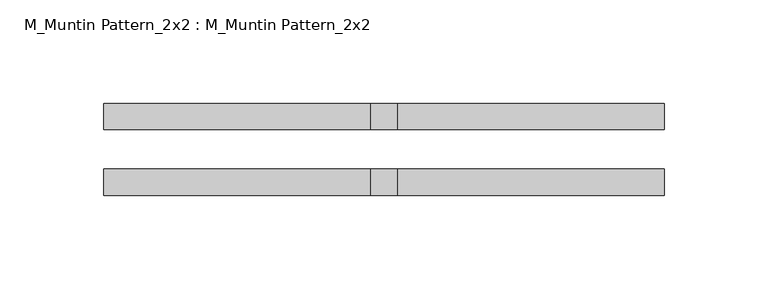
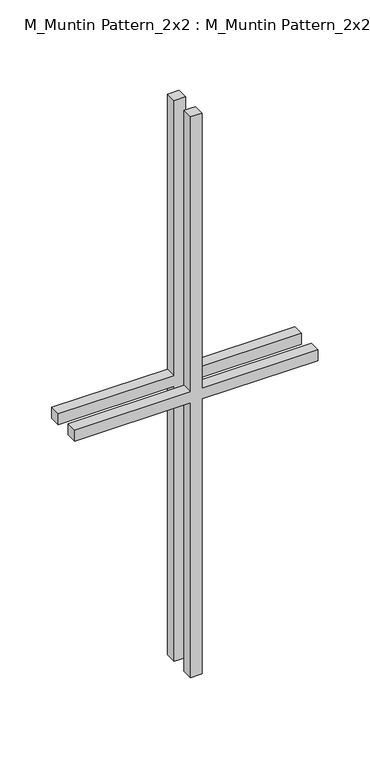
"""IFC4 building model written with IfcOpenShell, lengths in millimetres: proxy geometry, M_Muntin Pattern_2x2 : M_Muntin Pattern_2x2."""

from ifc_helpers import new_model, si_unit, frame, origin, place, context, project, spatial, polyline, outline, extrude, source, transform, mapped, element, save


def m_muntin_pattern_2x2_m_muntin_pattern_2x2_fa3d06ac(model_context):
    return source(origin(), model_context, "Body", "SweptSolid", [
        extrude(outline(polyline([(336.5, -6.35), (336.5, -135.4666667), (323.8, -135.4666667), (323.8, -6.35), (0.0, -6.35), (0.0, 6.35), (323.8, 6.35), (323.8, 135.4666667), (336.5, 135.4666667), (336.5, 6.35), (660.3, 6.35), (660.3, -6.35), (336.5, -6.35)])), frame((0.0, -22.225, 0.0), z_axis=(0.0, 1.0, 0.0), x_axis=(0.0, 0.0, 1.0)), (0.0, 0.0, 1.0), 12.7),
        extrude(outline(polyline([(336.5, -6.35), (336.5, -135.4666667), (323.8, -135.4666667), (323.8, -6.35), (0.0, -6.35), (0.0, 6.35), (323.8, 6.35), (323.8, 135.4666667), (336.5, 135.4666667), (336.5, 6.35), (660.3, 6.35), (660.3, -6.35), (336.5, -6.35)])), frame((0.0, 9.525, 0.0), z_axis=(0.0, 1.0, 0.0), x_axis=(0.0, 0.0, 1.0)), (0.0, 0.0, 1.0), 12.7),
    ])


if __name__ == "__main__":
    model = new_model("IFC4")
    model_context = context("Model", 3, world=origin())
    ifc_project = project(units=[si_unit("LENGTHUNIT", "METRE", prefix="MILLI")], contexts=[model_context])
    site = spatial("IfcSite", under=ifc_project)
    building = spatial("IfcBuilding", under=site)
    placement = place(None, origin())
    m_muntin_pattern_2x2_m_muntin_pattern_2x2_shape = m_muntin_pattern_2x2_m_muntin_pattern_2x2_fa3d06ac(model_context)
    element("IfcBuildingElementProxy", 1, Name="M_Muntin Pattern_2x2 : M_Muntin Pattern_2x2", ObjectType="M_Muntin Pattern_2x2 : M_Muntin Pattern_2x2", at=placement, inside=building, context=model_context, shape_type="MappedRepresentation", body=[
        mapped(m_muntin_pattern_2x2_m_muntin_pattern_2x2_shape, transform((0.0, 0.0, 0.0), x_axis=(1.0, 0.0, 0.0), y_axis=(0.0, 1.0, 0.0), z_axis=(0.0, 0.0, 1.0))),
    ])
    save(model, "model.ifc")

# Revit data of these elements
# Type "M_Muntin Pattern_2x2 : M_Muntin Pattern_2x2"
#   Width [instance default] = 3' - 11.24409"
#   Thickness = 0' - 0 1/2"
#   Height [instance default] = 3' - 11.24409"
#   Distance = 0' - 0 3/4"
#   Interior Material [instance default] = none
#   Exterior Material [instance default] = none
#   Default Elevation = 0
# Element 1 (IfcBuildingElementProxy, "M_Muntin Pattern_2x2 : M_Muntin Pattern_2x2")
#   Width = 0' - 10.66667"
#   Height = 2' - 1.99606"
#   Interior Material = Wood - Stained
#   Exterior Material = Clad - White
#   Materials on its faces: "Clad - White", "Wood - Stained"
# Materials
#   "Clad - White": class "Wood", colour RGB 242 242 238, transparency 0, Cost = 0
#   "Wood - Stained": class "Wood", colour RGB 224 178 126, transparency 0, Cost = 0
